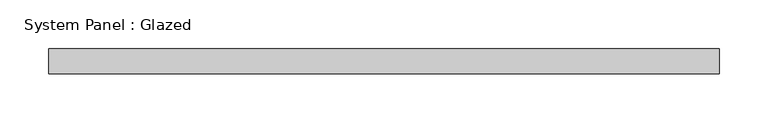
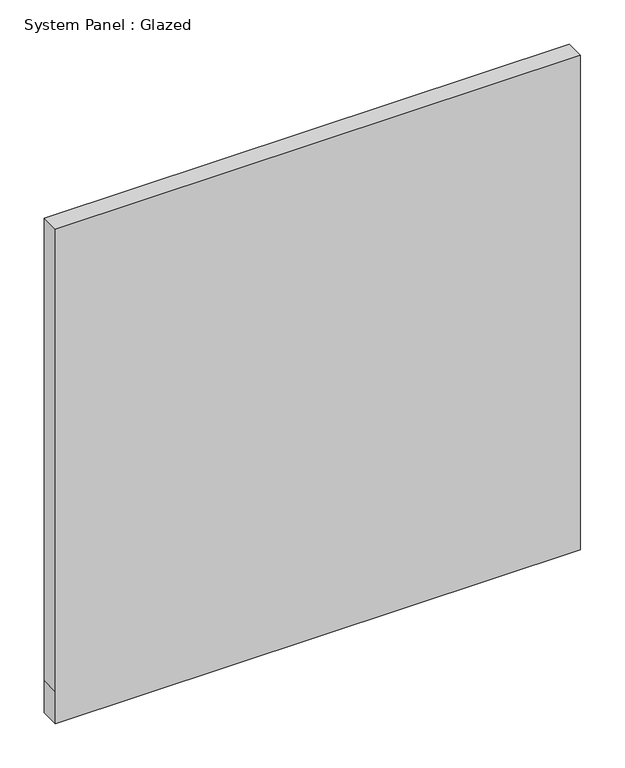
"""IFC4 building model written with IfcOpenShell, lengths in millimetres: plate geometry, System Panel : Glazed."""

from ifc_helpers import new_model, si_unit, frame, origin, place, context, project, spatial, polyline, outline, extrude, source, transform, mapped, element, save


def system_panel_glazed_af458955(model_context):
    return source(origin(), model_context, "Body", "SweptSolid", [
        extrude(outline(polyline([(0.0, -342.9727679), (0.0, 342.9727679), (44.45, 342.9727679), (683.176051, 342.9727679), (683.176051, -342.9727679), (44.45, -342.9727679), (0.0, -342.9727679)])), frame((0.0, 19.05, 0.0), z_axis=(0.0, 1.0, 0.0), x_axis=(0.0, 0.0, 1.0)), (0.0, 0.0, 1.0), 25.4),
    ])


if __name__ == "__main__":
    model = new_model("IFC4")
    model_context = context("Model", 3, world=origin())
    ifc_project = project(units=[si_unit("LENGTHUNIT", "METRE", prefix="MILLI")], contexts=[model_context])
    site = spatial("IfcSite", under=ifc_project)
    building = spatial("IfcBuilding", under=site)
    placement = place(None, origin())
    system_panel_glazed_shape = system_panel_glazed_af458955(model_context)
    element("IfcPlate", 1, ObjectType="System Panel : Glazed", at=placement, inside=building, context=model_context, shape_type="MappedRepresentation", body=[
        mapped(system_panel_glazed_shape, transform((0.0, 0.0, 0.0), x_axis=(1.0, 0.0, 0.0), y_axis=(0.0, 1.0, 0.0), z_axis=(0.0, 0.0, 1.0))),
    ])
    save(model, "model.ifc")

# Revit data of these elements
# Type "System Panel : Glazed"
#   Construction Type Id = "GSP4R"
#   Analytic Construction = "1/8 in Pilkington single glazing"
#   Visual Light Transmittance = 0.9
#   Solar Heat Gain Coefficient = 0.86
#   Heat Transfer Coefficient (U) = 1.18115 BTU/(h·ft²·°F)
#   Define Thermal Properties by = 1
# Element 1 (IfcPlate, "System Panel : Glazed")
#   Materials on its faces: "Glass"
# Materials
#   "Glass": class "Glass", colour RGB 0 128 192, transparency 0.75, Description = "Soda Lime Glass", Cost = 0
